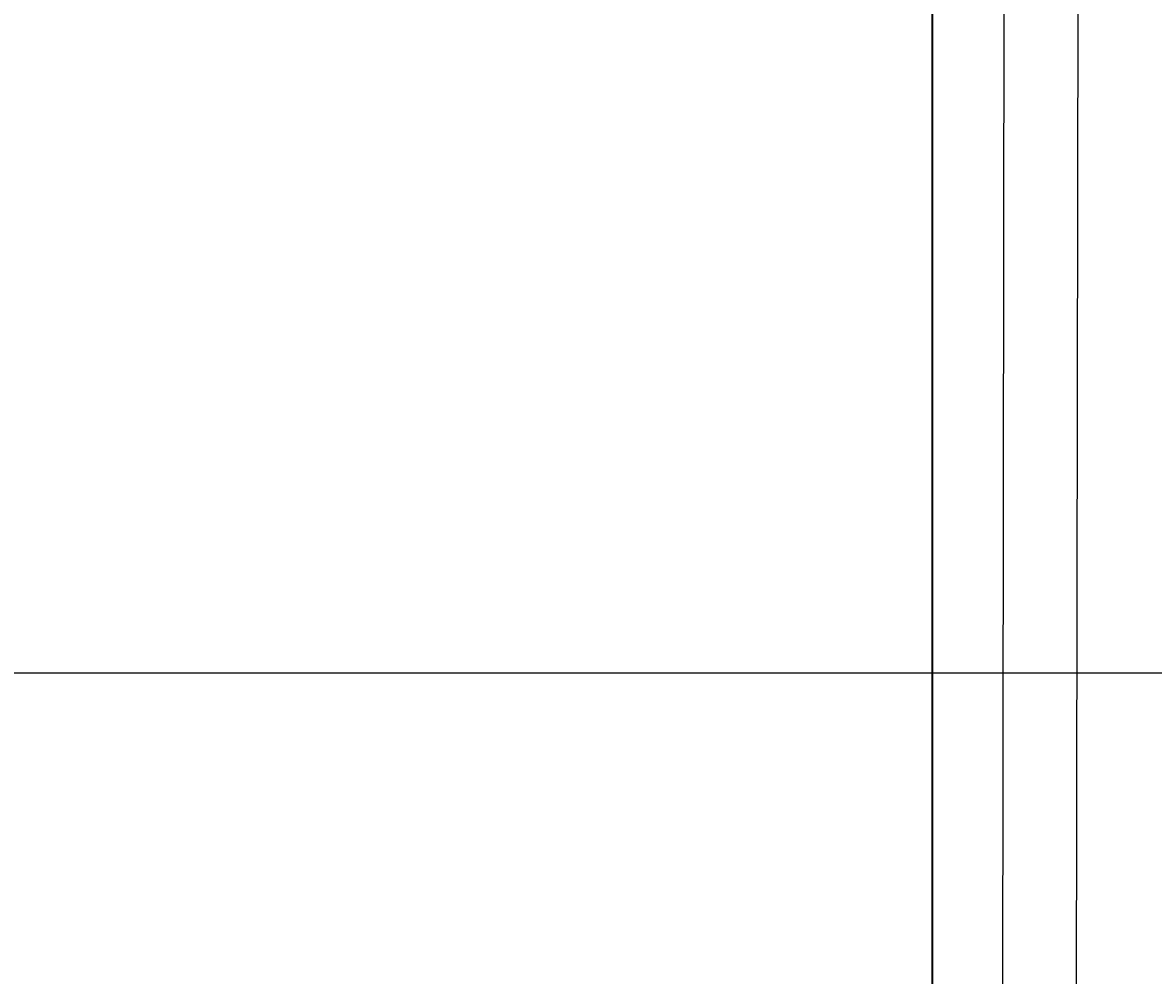
# Model space of a CAD drawing. Units: inches. Extents: x -301 to 715, y -607 to 364.
# Tile 19 of 141: x -66 to -35, y -448 to -422. Entities that reach past the tile are written whole.
import ezdxf

# ---------------------------------------------------------------- set-up
doc = ezdxf.new("R2010")
doc.units = ezdxf.units.IN
doc.header["$MEASUREMENT"] = 0
for name, color, linetype, lineweight in [('A-ANNO-DIMS', 2, 'Continuous', 18), ('A-DOOR', 4, 'Continuous', 25), ('A-SECT', 1, 'Continuous', 35)]:
    doc.layers.add(name, color=color, linetype=linetype, lineweight=lineweight)
doc.styles.get("Standard").update_dxf_attribs({"font": 'arial.ttf'})
doc.dimstyles.get("Standard").update_dxf_attribs({"dimtxt": 0.18, "dimasz": 0.18, "dimexe": 0.18, "dimexo": 0.0625, "dimgap": 0.09, "dimtad": 0, "dimtih": 1, "dimtoh": 1, "dimdec": 1, "dimzin": 0, "dimdsep": 46, "dimlunit": 4, "dimtxsty": 'Standard', "dimcen": 0.09, "dimclrd": 3, "dimclre": 4, "dimclrt": 6, "dimadec": 0, "dimazin": 0, "dimtfac": 1, "dimtdec": 1, "dimtofl": 0, "dimtmove": 0, "dimatfit": 3, "dimfxl": 1, "dimtfill": 2, "dimtfillclr": 51, "dimtolj": 1, "dimtzin": 0, "dimarcsym": 0})

# ---------------------------------------------------------------- blocks, each defined once
blk = doc.blocks.new('*D179')
at = {"layer": 'A-ANNO-DIMS', "color": 4, "lineweight": -2, "transparency": 16777216}
for p, q in [((-87.981, -433.54), (-87.981, -573.809)), ((-35.282, -463.54), (-35.282, -573.809))]:
    blk.add_line(p, q, dxfattribs=at)
at = {"layer": 'A-ANNO-DIMS', "color": 3, "lineweight": -2, "transparency": 16777216}
for p, q in [((-87.801, -573.629), (-62.174, -573.629)), ((-35.462, -573.629), (-61.089, -573.629))]:
    blk.add_line(p, q, dxfattribs=at)
at = {"layer": 'A-ANNO-DIMS', "color": 3, "transparency": 16777216}
for points in [[(-87.801, -573.599), (-87.801, -573.659), (-87.981, -573.629)], [(-35.462, -573.599), (-35.462, -573.659), (-35.282, -573.629)]]:
    blk.add_solid(points, dxfattribs=at)
at = {"layer": 'Defpoints', "color": 0, "transparency": 16777216}
for p in [(-87.981, -433.477), (-35.282, -463.477), (-35.282, -573.629)]:
    blk.add_point(p, dxfattribs=at)
at = {"layer": 'A-ANNO-DIMS', "color": 6, "transparency": 16777216, "insert": (-61.631, -573.629), "char_height": 0.18, "attachment_point": 5, "bg_fill": 1, "box_fill_scale": 1.25, "bg_fill_color": 51, "bg_fill_transparency": 0}
blk.add_mtext('\\A1;4\'-4 1/2"', dxfattribs=at)
blk = doc.blocks.new('*D187')
at = {"layer": 'A-ANNO-DIMS', "color": 4, "lineweight": -2, "transparency": 16777216}
for p, q in [((139.674, -385.477), (-266.112, -385.477)), ((143.155, -439.477), (-266.112, -439.477))]:
    blk.add_line(p, q, dxfattribs=at)
at = {"layer": 'A-ANNO-DIMS', "color": 3, "lineweight": -2, "transparency": 16777216}
for p, q in [((-265.932, -385.657), (-265.932, -412.296)), ((-265.932, -439.297), (-265.932, -412.659))]:
    blk.add_line(p, q, dxfattribs=at)
at = {"layer": 'A-ANNO-DIMS', "color": 3, "transparency": 16777216}
for points in [[(-265.962, -385.657), (-265.902, -385.657), (-265.932, -385.477)], [(-265.962, -439.297), (-265.902, -439.297), (-265.932, -439.477)]]:
    blk.add_solid(points, dxfattribs=at)
at = {"layer": 'Defpoints', "color": 0, "transparency": 16777216}
for p in [(-265.932, -385.477), (139.737, -385.477), (143.218, -439.477)]:
    blk.add_point(p, dxfattribs=at)
at = {"layer": 'A-ANNO-DIMS', "color": 6, "transparency": 16777216, "insert": (-265.932, -412.477), "char_height": 0.18, "attachment_point": 5, "bg_fill": 1, "box_fill_scale": 1.25, "bg_fill_color": 51, "bg_fill_transparency": 0}
blk.add_mtext('\\A1;4\'-6"', dxfattribs=at)

msp = doc.modelspace()

# ---------------------------------------------------------------- linework, layer by layer
at = {"layer": 'A-DOOR'}
for p, q in [((-39.282, -385.476), (-39.396, -463.476)), ((-37.282, -385.479), (-37.396, -463.479))]:
    msp.add_line(p, q, dxfattribs=at)
at = {"layer": 'A-SECT'}
msp.add_line((-41.282, -361.477), (-41.282, -481.477), dxfattribs=at)

# ---------------------------------------------------------------- dimensions: what is measured, and where the dimension line sits
at = {"layer": 'A-ANNO-DIMS'}
dim = msp.add_linear_dim(base=(-265.932, -385.477), p1=(143.218, -439.477), p2=(139.737, -385.477), angle=90, dimstyle='Standard', override={"dimdec": 1, "dimlfac": 1, "dimrnd": 0, "dimzin": 1, "dimdsep": 46, "dimlunit": 4, "dimfrac": 2}, dxfattribs=at)
dim.commit()
dim.dimension.update_dxf_attribs({"geometry": '*D187', "text_midpoint": (-265.932, -412.477)})
dim = msp.add_linear_dim(base=(-35.282, -573.629), p1=(-87.981, -433.477), p2=(-35.282, -463.477), dimstyle='Standard', override={"dimdec": 1, "dimlfac": 1, "dimrnd": 0, "dimzin": 1, "dimdsep": 46, "dimlunit": 4, "dimfrac": 2}, dxfattribs=at)
dim.commit()
dim.dimension.update_dxf_attribs({"geometry": '*D179', "text_midpoint": (-61.631, -573.629)})

doc.saveas('drawing.dxf')
